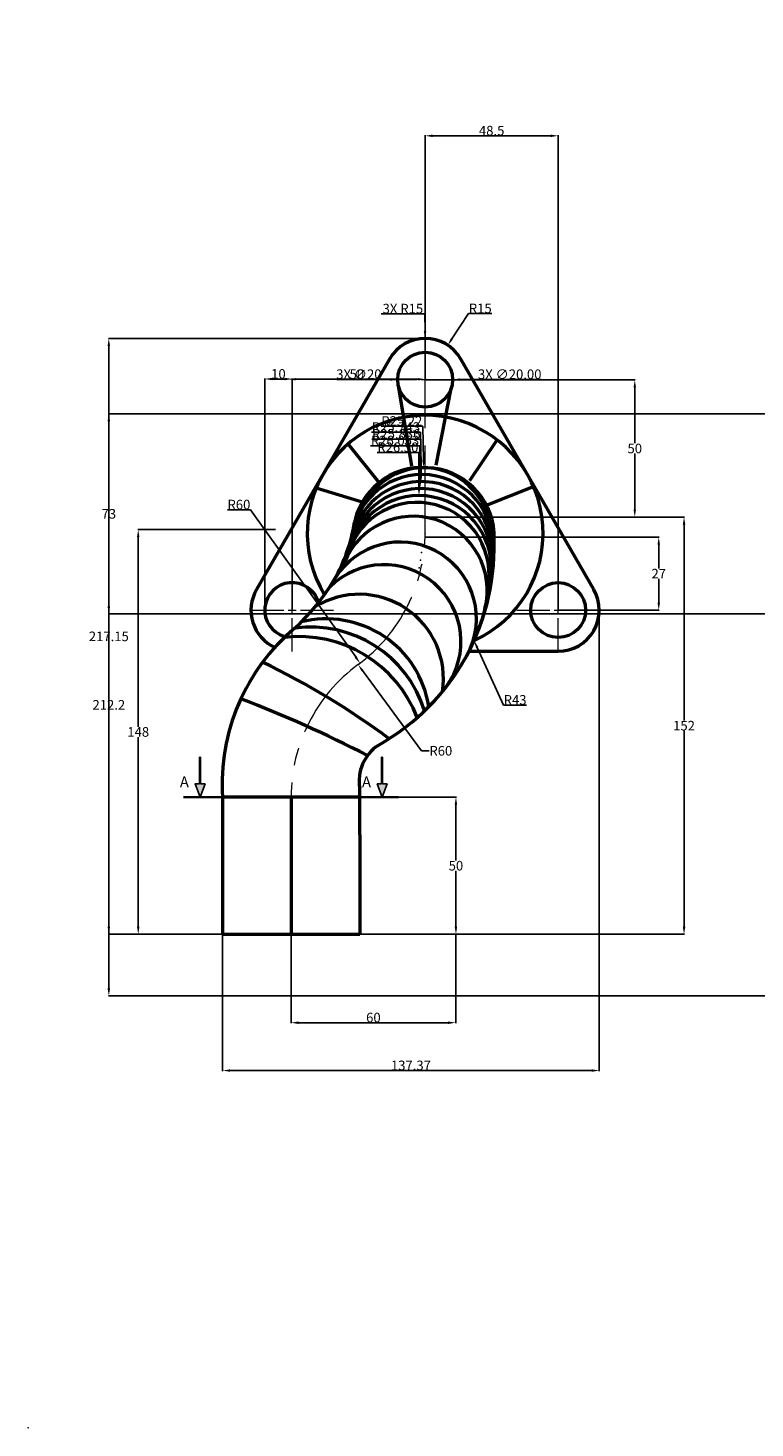
# Model space of a CAD drawing. Units: millimetres. Extents: x 795 to 1506, y 326 to 837.
# Tile 1 of 2: x 795 to 1060, y 326 to 837. Entities that reach past the tile are written whole.
import ezdxf

# ---------------------------------------------------------------- set-up
doc = ezdxf.new("R2010")
doc.units = ezdxf.units.MM
doc.header["$MEASUREMENT"] = 0
doc.linetypes.add('CENTER', pattern=[50.8, 31.75, -6.35, 6.35, -6.35])
doc.linetypes.add('PHANTOM', pattern=[63.5, 31.75, -6.35, 6.35, -6.35, 6.35, -6.35])
for name, color, linetype, lineweight in [('M-CNTR', 251, 'CENTER', 18), ('M-DIMS', 2, 'Continuous', 25), ('M-OUTL', 7, 'Continuous', 50), ('M-SECT', 7, 'PHANTOM', 35), ('M-SYMB', 7, 'Continuous', 25), ('M-TEXT', 7, 'Continuous', 25)]:
    doc.layers.add(name, color=color, linetype=linetype, lineweight=lineweight)
doc.styles.get("Standard").update_dxf_attribs({"font": 'arial.ttf'})
doc.dimstyles.get("Standard").update_dxf_attribs({"dimtxt": 3.5, "dimasz": 2.75, "dimexe": 0.18, "dimexo": 0.0625, "dimgap": 0.09, "dimtad": 1, "dimtih": 1, "dimtoh": 1, "dimdec": 0, "dimzin": 0, "dimdsep": 46, "dimtxsty": 'Standard', "dimcen": 0.09, "dimadec": 0, "dimazin": 0, "dimtfac": 1, "dimtdec": 0, "dimtofl": 0, "dimtmove": 0, "dimatfit": 3, "dimfxl": 1, "dimtolj": 1, "dimtzin": 0, "dimarcsym": 0})

# ---------------------------------------------------------------- blocks, each defined once
blk = doc.blocks.new('*U1')
at = {"layer": 'M-CNTR', "color": 0, "transparency": 16777216}
for p, q in [((0, 3), (0, 15.12)), ((-15.12, 0), (-3, 0)), ((3, 0), (15.12, 0)), ((0, -15.12), (0, -3))]:
    blk.add_line(p, q, dxfattribs=at)
at = {"layer": 'M-CNTR', "color": 0, "linetype": 'Continuous', "transparency": 16777216}
for p, q in [((-1.5, 0), (1.5, 0)), ((0, -1.5), (0, 1.5))]:
    blk.add_line(p, q, dxfattribs=at)
blk = doc.blocks.new('*U2')
at = {"layer": 'M-CNTR', "color": 0, "transparency": 16777216}
for p, q in [((0, 3), (0, 15.12)), ((-15.12, 0), (-3, 0)), ((3, 0), (15.12, 0)), ((0, -15.12), (0, -3))]:
    blk.add_line(p, q, dxfattribs=at)
at = {"layer": 'M-CNTR', "color": 0, "linetype": 'Continuous', "transparency": 16777216}
for p, q in [((-1.5, 0), (1.5, 0)), ((0, -1.5), (0, 1.5))]:
    blk.add_line(p, q, dxfattribs=at)
blk = doc.blocks.new('*U3')
at = {"layer": 'M-CNTR', "color": 0, "transparency": 16777216}
for p, q in [((0, 3), (0, 15.12)), ((-15.12, 0), (-3, 0)), ((3, 0), (15.12, 0)), ((0, -15.12), (0, -3))]:
    blk.add_line(p, q, dxfattribs=at)
at = {"layer": 'M-CNTR', "color": 0, "linetype": 'Continuous', "transparency": 16777216}
for p, q in [((-1.5, 0), (1.5, 0)), ((0, -1.5), (0, 1.5))]:
    blk.add_line(p, q, dxfattribs=at)
blk = doc.blocks.new('*D8')
at = {"layer": 'Defpoints', "color": 0, "transparency": 16777216}
for p in [(834.94, 653.74), (885.07, 653.74), (865.68, 506.24)]:
    blk.add_point(p, dxfattribs=at)
at = {"layer": 'M-DIMS', "color": 0, "lineweight": -2, "transparency": 16777216}
for p, q in [((885, 653.74), (834.76, 653.74)), ((834.94, 650.99), (834.94, 581.87)), ((834.94, 508.99), (834.94, 578.12)), ((865.61, 506.24), (834.76, 506.24))]:
    blk.add_line(p, q, dxfattribs=at)
at = {"layer": 'M-DIMS', "color": 0, "transparency": 16777216}
for points in [[(834.49, 650.99), (835.4, 650.99), (834.94, 653.74)], [(834.49, 508.99), (835.4, 508.99), (834.94, 506.24)]]:
    blk.add_solid(points, dxfattribs=at)
at = {"layer": 'M-DIMS', "color": 0, "transparency": 16777216, "insert": (834.94, 579.99), "char_height": 3.5, "attachment_point": 5}
blk.add_mtext('\\A1;148', dxfattribs=at)
blk = doc.blocks.new('*D9')
at = {"layer": 'Defpoints', "color": 0, "transparency": 16777216}
for p in [(881.05, 708.62), (881.05, 624.39), (891.05, 624.39)]:
    blk.add_point(p, dxfattribs=at)
at = {"layer": 'M-DIMS', "color": 0, "lineweight": -2, "transparency": 16777216}
for p, q in [((881.05, 624.46), (881.05, 708.8)), ((888.3, 708.62), (883.8, 708.62)), ((891.05, 624.46), (891.05, 708.8))]:
    blk.add_line(p, q, dxfattribs=at)
at = {"layer": 'M-DIMS', "color": 0, "transparency": 16777216}
for points in [[(883.8, 709.07), (883.8, 708.16), (881.05, 708.62)], [(888.3, 709.07), (888.3, 708.16), (891.05, 708.62)]]:
    blk.add_solid(points, dxfattribs=at)
at = {"layer": 'M-DIMS', "color": 0, "transparency": 16777216, "insert": (886.05, 710.49), "char_height": 3.5, "attachment_point": 5}
blk.add_mtext('\\A1;10', dxfattribs=at)
blk = doc.blocks.new('*D10')
at = {"layer": 'Defpoints', "color": 0, "transparency": 16777216}
for p in [(947.78, 720.93), (939.55, 708.39)]:
    blk.add_point(p, dxfattribs=at)
at = {"layer": 'M-DIMS', "color": 0, "lineweight": -2, "transparency": 16777216}
for p, q in [((955.36, 732.49), (949.29, 723.23)), ((963.84, 732.49), (955.36, 732.49)), ((939.46, 708.39), (939.64, 708.39)), ((939.55, 708.3), (939.55, 708.48))]:
    blk.add_line(p, q, dxfattribs=at)
at = {"layer": 'M-DIMS', "color": 0, "transparency": 16777216}
blk.add_solid([(948.9, 723.48), (949.67, 722.98), (947.78, 720.93)], dxfattribs=at)
at = {"layer": 'M-DIMS', "color": 0, "transparency": 16777216, "insert": (959.64, 734.36), "char_height": 3.5, "attachment_point": 5}
blk.add_mtext('\\A1;R15', dxfattribs=at)
blk = doc.blocks.new('*D11')
at = {"layer": 'Defpoints', "color": 0, "transparency": 16777216}
for p in [(889.64, 708.52), (889.64, 708.39), (939.64, 708.39)]:
    blk.add_point(p, dxfattribs=at)
at = {"layer": 'M-DIMS', "color": 0, "lineweight": -2, "transparency": 16777216}
for p, q in [((889.64, 708.46), (889.64, 708.7)), ((936.89, 708.52), (892.39, 708.52)), ((939.64, 708.46), (939.64, 708.7))]:
    blk.add_line(p, q, dxfattribs=at)
at = {"layer": 'M-DIMS', "color": 0, "transparency": 16777216}
for points in [[(892.39, 708.98), (892.39, 708.06), (889.64, 708.52)], [(936.89, 708.98), (936.89, 708.06), (939.64, 708.52)]]:
    blk.add_solid(points, dxfattribs=at)
at = {"layer": 'M-DIMS', "color": 0, "transparency": 16777216, "insert": (914.64, 710.4), "char_height": 3.5, "attachment_point": 5}
blk.add_mtext('\\A1;50', dxfattribs=at)
blk = doc.blocks.new('*D12')
at = {"layer": 'Defpoints', "color": 0, "transparency": 16777216}
for p in [(915.08, 604.54), (950.68, 556.24)]:
    blk.add_point(p, dxfattribs=at)
at = {"layer": 'M-DIMS', "color": 0, "lineweight": -2, "transparency": 16777216}
for p, q in [((938.24, 573.11), (916.71, 602.33)), ((940.99, 573.11), (938.24, 573.11))]:
    blk.add_line(p, q, dxfattribs=at)
at = {"layer": 'M-DIMS', "color": 0, "transparency": 16777216}
blk.add_solid([(917.08, 602.6), (916.34, 602.06), (915.08, 604.54)], dxfattribs=at)
at = {"layer": 'M-DIMS', "color": 0, "transparency": 16777216, "insert": (945.26, 573.11), "char_height": 3.5, "attachment_point": 5}
blk.add_mtext('\\A1;R60', dxfattribs=at)
blk = doc.blocks.new('*D13')
at = {"layer": 'Defpoints', "color": 0, "transparency": 16777216}
for p in [(939.52, 650.96), (1024.71, 650.96), (988.04, 624.39)]:
    blk.add_point(p, dxfattribs=at)
at = {"layer": 'M-DIMS', "color": 0, "lineweight": -2, "transparency": 16777216}
for p, q in [((939.58, 650.96), (1024.89, 650.96)), ((1024.71, 648.21), (1024.71, 639.52)), ((1024.71, 627.14), (1024.71, 635.83)), ((988.11, 624.39), (1024.89, 624.39))]:
    blk.add_line(p, q, dxfattribs=at)
at = {"layer": 'M-DIMS', "color": 0, "transparency": 16777216}
for points in [[(1024.25, 648.21), (1025.17, 648.21), (1024.71, 650.96)], [(1024.25, 627.14), (1025.17, 627.14), (1024.71, 624.39)]]:
    blk.add_solid(points, dxfattribs=at)
at = {"layer": 'M-DIMS', "color": 0, "transparency": 16777216, "insert": (1024.71, 637.68), "char_height": 3.5, "attachment_point": 5}
blk.add_mtext('\\A1;27', dxfattribs=at)
blk = doc.blocks.new('*D14')
at = {"layer": 'Defpoints', "color": 0, "transparency": 16777216}
for p in [(939.55, 708.3), (939.55, 658.3), (1015.97, 658.3)]:
    blk.add_point(p, dxfattribs=at)
at = {"layer": 'M-DIMS', "color": 0, "lineweight": -2, "transparency": 16777216}
for p, q in [((939.61, 708.3), (1016.15, 708.3)), ((1015.97, 705.55), (1015.97, 685.18)), ((1015.97, 661.05), (1015.97, 681.43)), ((939.61, 658.3), (1016.15, 658.3))]:
    blk.add_line(p, q, dxfattribs=at)
at = {"layer": 'M-DIMS', "color": 0, "transparency": 16777216}
for points in [[(1015.51, 705.55), (1016.42, 705.55), (1015.97, 708.3)], [(1015.51, 661.05), (1016.42, 661.05), (1015.97, 658.3)]]:
    blk.add_solid(points, dxfattribs=at)
at = {"layer": 'M-DIMS', "color": 0, "transparency": 16777216, "insert": (1015.97, 683.3), "char_height": 3.5, "attachment_point": 5}
blk.add_mtext('\\A1;50', dxfattribs=at)
blk = doc.blocks.new('*D15')
at = {"layer": 'Defpoints', "color": 0, "transparency": 16777216}
for p in [(939.55, 658.3), (950.68, 506.24), (1033.93, 506.24)]:
    blk.add_point(p, dxfattribs=at)
at = {"layer": 'M-DIMS', "color": 0, "lineweight": -2, "transparency": 16777216}
for p, q in [((939.61, 658.3), (1034.11, 658.3)), ((1033.93, 655.55), (1033.93, 584.15)), ((1033.93, 508.99), (1033.93, 580.4)), ((950.74, 506.24), (1034.11, 506.24))]:
    blk.add_line(p, q, dxfattribs=at)
at = {"layer": 'M-DIMS', "color": 0, "transparency": 16777216}
for points in [[(1033.47, 655.55), (1034.39, 655.55), (1033.93, 658.3)], [(1033.47, 508.99), (1034.39, 508.99), (1033.93, 506.24)]]:
    blk.add_solid(points, dxfattribs=at)
at = {"layer": 'M-DIMS', "color": 0, "transparency": 16777216, "insert": (1033.93, 582.27), "char_height": 3.5, "attachment_point": 5}
blk.add_mtext('\\A1;152', dxfattribs=at)
blk = doc.blocks.new('*D18')
at = {"layer": 'Defpoints', "color": 0, "transparency": 16777216}
for p in [(890.68, 506.24), (950.68, 506.24), (950.68, 474)]:
    blk.add_point(p, dxfattribs=at)
at = {"layer": 'M-DIMS', "color": 0, "lineweight": -2, "transparency": 16777216}
for p, q in [((890.68, 506.18), (890.68, 473.82)), ((950.68, 506.18), (950.68, 473.82)), ((893.43, 474), (947.93, 474))]:
    blk.add_line(p, q, dxfattribs=at)
at = {"layer": 'M-DIMS', "color": 0, "transparency": 16777216}
for points in [[(893.43, 474.46), (893.43, 473.54), (890.68, 474)], [(947.93, 474.46), (947.93, 473.54), (950.68, 474)]]:
    blk.add_solid(points, dxfattribs=at)
at = {"layer": 'M-DIMS', "color": 0, "transparency": 16777216, "insert": (920.68, 475.88), "char_height": 3.5, "attachment_point": 5}
blk.add_mtext('\\A1;60', dxfattribs=at)
blk = doc.blocks.new('*D19')
at = {"layer": 'Defpoints', "color": 0, "transparency": 16777216}
for p in [(915.81, 605.08), (950.68, 556.24)]:
    blk.add_point(p, dxfattribs=at)
at = {"layer": 'M-DIMS', "color": 0, "lineweight": -2, "transparency": 16777216}
for p, q in [((867.47, 660.97), (875.91, 660.97)), ((875.91, 660.97), (914.22, 607.32)), ((950.59, 556.24), (950.77, 556.24)), ((950.68, 556.15), (950.68, 556.33))]:
    blk.add_line(p, q, dxfattribs=at)
blk.add_arc((950.68, 556.24), 60, 125.3513, 126.2918, dxfattribs=at)
at = {"layer": 'M-DIMS', "color": 0, "transparency": 16777216}
blk.add_solid([(914.59, 607.58), (913.84, 607.05), (915.81, 605.08)], dxfattribs=at)
at = {"layer": 'M-DIMS', "color": 0, "transparency": 16777216, "insert": (871.65, 662.85), "char_height": 3.5, "attachment_point": 5}
blk.add_mtext('\\A1;R60', dxfattribs=at)
blk = doc.blocks.new('*D20')
at = {"layer": 'Defpoints', "color": 0, "transparency": 16777216}
for p in [(915.68, 556.24), (950.77, 556.24), (915.68, 506.24)]:
    blk.add_point(p, dxfattribs=at)
at = {"layer": 'M-DIMS', "color": 0, "lineweight": -2, "transparency": 16777216}
for p, q in [((915.74, 556.24), (950.95, 556.24)), ((950.77, 553.49), (950.77, 533.12)), ((950.77, 508.99), (950.77, 529.37)), ((915.74, 506.24), (950.95, 506.24))]:
    blk.add_line(p, q, dxfattribs=at)
at = {"layer": 'M-DIMS', "color": 0, "transparency": 16777216}
for points in [[(950.31, 553.49), (951.22, 553.49), (950.77, 556.24)], [(950.31, 508.99), (951.22, 508.99), (950.77, 506.24)]]:
    blk.add_solid(points, dxfattribs=at)
at = {"layer": 'M-DIMS', "color": 0, "transparency": 16777216, "insert": (950.77, 531.24), "char_height": 3.5, "attachment_point": 5}
blk.add_mtext('\\A1;50', dxfattribs=at)
blk = doc.blocks.new('*D21')
at = {"layer": 'Defpoints', "color": 0, "transparency": 16777216}
for p in [(988.04, 797.27), (939.55, 708.39), (988.04, 624.39)]:
    blk.add_point(p, dxfattribs=at)
at = {"layer": 'M-DIMS', "color": 0, "lineweight": -2, "transparency": 16777216}
for p, q in [((939.55, 708.46), (939.55, 797.45)), ((942.3, 797.27), (985.29, 797.27)), ((988.04, 624.46), (988.04, 797.45))]:
    blk.add_line(p, q, dxfattribs=at)
at = {"layer": 'M-DIMS', "color": 0, "transparency": 16777216}
for points in [[(942.3, 797.72), (942.3, 796.81), (939.55, 797.27)], [(985.29, 797.72), (985.29, 796.81), (988.04, 797.27)]]:
    blk.add_solid(points, dxfattribs=at)
at = {"layer": 'M-DIMS', "color": 0, "transparency": 16777216, "insert": (963.8, 799.14), "char_height": 3.5, "attachment_point": 5}
blk.add_mtext('\\A1;48.5', dxfattribs=at)
blk = doc.blocks.new('*D22')
at = {"layer": 'Defpoints', "color": 0, "transparency": 16777216}
for p in [(1003.04, 624.39), (865.68, 506.24), (1003.04, 456.57)]:
    blk.add_point(p, dxfattribs=at)
at = {"layer": 'M-DIMS', "color": 0, "lineweight": -2, "transparency": 16777216}
for p, q in [((1003.04, 624.33), (1003.04, 456.39)), ((865.68, 506.18), (865.68, 456.39)), ((868.43, 456.57), (1000.29, 456.57))]:
    blk.add_line(p, q, dxfattribs=at)
at = {"layer": 'M-DIMS', "color": 0, "transparency": 16777216}
for points in [[(868.43, 457.02), (868.43, 456.11), (865.68, 456.57)], [(1000.29, 457.02), (1000.29, 456.11), (1003.04, 456.57)]]:
    blk.add_solid(points, dxfattribs=at)
at = {"layer": 'M-DIMS', "color": 0, "transparency": 16777216, "insert": (934.36, 458.44), "char_height": 3.5, "attachment_point": 5}
blk.add_mtext('\\A1;137.37', dxfattribs=at)
blk = doc.blocks.new('*D23')
at = {"layer": 'Defpoints', "color": 0, "transparency": 16777216}
for p in [(824.22, 723.39), (939.55, 723.39), (865.68, 506.24)]:
    blk.add_point(p, dxfattribs=at)
at = {"layer": 'M-DIMS', "color": 0, "lineweight": -2, "transparency": 16777216}
for p, q in [((939.48, 723.39), (824.04, 723.39)), ((824.22, 720.64), (824.22, 616.7)), ((824.22, 508.99), (824.22, 612.94)), ((865.61, 506.24), (824.04, 506.24))]:
    blk.add_line(p, q, dxfattribs=at)
at = {"layer": 'M-DIMS', "color": 0, "transparency": 16777216}
for points in [[(823.76, 720.64), (824.68, 720.64), (824.22, 723.39)], [(823.76, 508.99), (824.68, 508.99), (824.22, 506.24)]]:
    blk.add_solid(points, dxfattribs=at)
at = {"layer": 'M-DIMS', "color": 0, "transparency": 16777216, "insert": (824.22, 614.82), "char_height": 3.5, "attachment_point": 5}
blk.add_mtext('\\A1;217.15', dxfattribs=at)
blk = doc.blocks.new('*D25')
at = {"layer": 'Defpoints', "color": 0, "transparency": 16777216}
for p in [(1310.11, 695.98), (824.22, 622.98), (1265.11, 622.98)]:
    blk.add_point(p, dxfattribs=at)
at = {"layer": 'M-DIMS', "color": 0, "lineweight": -2, "transparency": 16777216}
for p, q in [((1310.05, 695.98), (824.04, 695.98)), ((824.22, 693.23), (824.22, 661.36)), ((824.22, 625.73), (824.22, 657.6)), ((1265.05, 622.98), (824.04, 622.98))]:
    blk.add_line(p, q, dxfattribs=at)
at = {"layer": 'M-DIMS', "color": 0, "transparency": 16777216}
for points in [[(823.76, 693.23), (824.68, 693.23), (824.22, 695.98)], [(823.76, 625.73), (824.68, 625.73), (824.22, 622.98)]]:
    blk.add_solid(points, dxfattribs=at)
at = {"layer": 'M-DIMS', "color": 0, "transparency": 16777216, "insert": (824.22, 659.48), "char_height": 3.5, "attachment_point": 5}
blk.add_mtext('\\A1;73', dxfattribs=at)
blk = doc.blocks.new('*D27')
at = {"layer": 'Defpoints', "color": 0, "transparency": 16777216}
for p in [(824.22, 695.98), (1310.11, 695.98), (1165.11, 483.77)]:
    blk.add_point(p, dxfattribs=at)
at = {"layer": 'M-DIMS', "color": 0, "lineweight": -2, "transparency": 16777216}
for p, q in [((1310.05, 695.98), (824.04, 695.98)), ((824.22, 693.23), (824.22, 591.72)), ((824.22, 486.52), (824.22, 588.03)), ((1165.05, 483.77), (824.04, 483.77))]:
    blk.add_line(p, q, dxfattribs=at)
at = {"layer": 'M-DIMS', "color": 0, "transparency": 16777216}
for points in [[(823.76, 693.23), (824.68, 693.23), (824.22, 695.98)], [(823.76, 486.52), (824.68, 486.52), (824.22, 483.77)]]:
    blk.add_solid(points, dxfattribs=at)
at = {"layer": 'M-DIMS', "color": 0, "transparency": 16777216, "insert": (824.22, 589.87), "char_height": 3.5, "attachment_point": 5}
blk.add_mtext('\\A1;212.2', dxfattribs=at)
blk = doc.blocks.new('*D30')
at = {"layer": 'Defpoints', "color": 0, "transparency": 16777216}
for p in [(939.5, 723.39), (939.55, 708.39)]:
    blk.add_point(p, dxfattribs=at)
at = {"layer": 'M-DIMS', "color": 0, "lineweight": -2, "transparency": 16777216}
for p, q in [((923.47, 732.39), (939.47, 732.39)), ((939.47, 732.39), (939.49, 726.14)), ((939.46, 708.39), (939.64, 708.39)), ((939.55, 708.3), (939.55, 708.48))]:
    blk.add_line(p, q, dxfattribs=at)
at = {"layer": 'M-DIMS', "color": 0, "transparency": 16777216}
blk.add_solid([(939.95, 726.14), (939.03, 726.14), (939.5, 723.39)], dxfattribs=at)
at = {"layer": 'M-DIMS', "color": 0, "transparency": 16777216, "insert": (931.43, 734.27), "char_height": 3.5, "attachment_point": 5}
blk.add_mtext('\\A1;3X R15', dxfattribs=at)
blk = doc.blocks.new('*D31')
at = {"layer": 'Defpoints', "color": 0, "transparency": 16777216}
for p in [(929.55, 708.4), (949.55, 708.39)]:
    blk.add_point(p, dxfattribs=at)
at = {"layer": 'M-DIMS', "color": 0, "lineweight": -2, "transparency": 16777216}
for p, q in [((907.32, 708.4), (923.55, 708.4)), ((923.55, 708.4), (926.8, 708.4)), ((939.46, 708.39), (939.64, 708.39)), ((939.55, 708.3), (939.55, 708.48))]:
    blk.add_line(p, q, dxfattribs=at)
at = {"layer": 'M-DIMS', "color": 0, "transparency": 16777216}
blk.add_solid([(926.8, 708.86), (926.8, 707.94), (929.55, 708.4)], dxfattribs=at)
at = {"layer": 'M-DIMS', "color": 0, "transparency": 16777216, "insert": (915.39, 710.38), "char_height": 3.5, "attachment_point": 5}
blk.add_mtext('\\A1;3X ∅20', dxfattribs=at)
blk = doc.blocks.new('*D32')
at = {"layer": 'Defpoints', "color": 0, "transparency": 16777216}
for p in [(939.55, 652.39), (957.37, 613.26)]:
    blk.add_point(p, dxfattribs=at)
at = {"layer": 'M-DIMS', "color": 0, "lineweight": -2, "transparency": 16777216}
for p, q in [((939.46, 652.39), (939.64, 652.39)), ((939.55, 652.3), (939.55, 652.48)), ((968.06, 589.78), (958.51, 610.76)), ((976.52, 589.78), (968.06, 589.78))]:
    blk.add_line(p, q, dxfattribs=at)
at = {"layer": 'M-DIMS', "color": 0, "transparency": 16777216}
blk.add_solid([(958.93, 610.95), (958.09, 610.57), (957.37, 613.26)], dxfattribs=at)
at = {"layer": 'M-DIMS', "color": 0, "transparency": 16777216, "insert": (972.34, 591.66), "char_height": 3.5, "attachment_point": 5}
blk.add_mtext('\\A1;R43', dxfattribs=at)
blk = doc.blocks.new('*D35')
at = {"layer": 'Defpoints', "color": 0, "transparency": 16777216}
for p in [(929.55, 708.4), (949.55, 708.39)]:
    blk.add_point(p, dxfattribs=at)
at = {"layer": 'M-DIMS', "color": 0, "lineweight": -2, "transparency": 16777216}
for p, q in [((939.46, 708.39), (939.64, 708.39)), ((939.55, 708.3), (939.55, 708.48)), ((958.82, 708.39), (952.3, 708.39)), ((981.85, 708.39), (958.82, 708.39))]:
    blk.add_line(p, q, dxfattribs=at)
at = {"layer": 'M-DIMS', "color": 0, "transparency": 16777216}
blk.add_solid([(952.3, 708.85), (952.3, 707.93), (949.55, 708.39)], dxfattribs=at)
at = {"layer": 'M-DIMS', "color": 0, "transparency": 16777216, "insert": (970.38, 710.36), "char_height": 3.5, "attachment_point": 5}
blk.add_mtext('\\A1;3X ∅20.00', dxfattribs=at)
blk = doc.blocks.new('*D38')
at = {"layer": 'Defpoints', "color": 0, "transparency": 16777216}
for p in [(1227.9, 642.63), (794.84, 326.38)]:
    blk.add_point(p, dxfattribs=at)
at = {"layer": 'M-DIMS', "color": 0, "lineweight": -2, "transparency": 16777216}
for p, q in [((1487.74, 832.38), (1230.12, 644.25)), ((1505.7, 832.38), (1487.74, 832.38)), ((794.75, 326.38), (794.93, 326.38)), ((794.84, 326.29), (794.84, 326.47))]:
    blk.add_line(p, q, dxfattribs=at)
at = {"layer": 'M-DIMS', "color": 0, "transparency": 16777216}
blk.add_solid([(1229.85, 644.62), (1230.39, 643.88), (1227.9, 642.63)], dxfattribs=at)
at = {"layer": 'M-DIMS', "color": 0, "transparency": 16777216, "insert": (1496.76, 834.26), "char_height": 3.5, "attachment_point": 5}
blk.add_mtext('\\A1;R536.24', dxfattribs=at)
blk = doc.blocks.new('*D48')
at = {"layer": 'Defpoints', "color": 0, "transparency": 16777216}
for p in [(939, 676.3), (939.53, 651.08)]:
    blk.add_point(p, dxfattribs=at)
at = {"layer": 'M-DIMS', "color": 0, "lineweight": -2, "transparency": 16777216}
for p, q in [((923.47, 691.43), (938.68, 691.43)), ((938.68, 691.43), (938.94, 679.05)), ((939.44, 651.08), (939.62, 651.08)), ((939.53, 650.99), (939.53, 651.17))]:
    blk.add_line(p, q, dxfattribs=at)
at = {"layer": 'M-DIMS', "color": 0, "transparency": 16777216}
blk.add_solid([(939.4, 679.06), (938.48, 679.04), (939, 676.3)], dxfattribs=at)
at = {"layer": 'M-DIMS', "color": 0, "transparency": 16777216, "insert": (931.03, 693.31), "char_height": 3.5, "attachment_point": 5}
blk.add_mtext('\\A1;R25.22', dxfattribs=at)
blk = doc.blocks.new('*D49')
at = {"layer": 'Defpoints', "color": 0, "transparency": 16777216}
for p in [(938.1, 673.79), (938.41, 648.05)]:
    blk.add_point(p, dxfattribs=at)
at = {"layer": 'M-DIMS', "color": 0, "lineweight": -2, "transparency": 16777216}
for p, q in [((919.94, 689.23), (937.91, 689.23)), ((937.91, 689.23), (938.07, 676.54)), ((938.32, 648.05), (938.5, 648.05)), ((938.41, 647.96), (938.41, 648.14))]:
    blk.add_line(p, q, dxfattribs=at)
at = {"layer": 'M-DIMS', "color": 0, "transparency": 16777216}
blk.add_solid([(938.53, 676.54), (937.61, 676.53), (938.1, 673.79)], dxfattribs=at)
at = {"layer": 'M-DIMS', "color": 0, "transparency": 16777216, "insert": (928.88, 691.11), "char_height": 3.5, "attachment_point": 5}
blk.add_mtext('\\A1;R25.743', dxfattribs=at)
blk = doc.blocks.new('*D50')
at = {"layer": 'Defpoints', "color": 0, "transparency": 16777216}
for p in [(938.1, 671.22), (938.22, 645.38)]:
    blk.add_point(p, dxfattribs=at)
at = {"layer": 'M-DIMS', "color": 0, "lineweight": -2, "transparency": 16777216}
for p, q in [((920.06, 686.72), (938.02, 686.72)), ((938.02, 686.72), (938.09, 673.97)), ((938.13, 645.38), (938.31, 645.38)), ((938.22, 645.29), (938.22, 645.47))]:
    blk.add_line(p, q, dxfattribs=at)
at = {"layer": 'M-DIMS', "color": 0, "transparency": 16777216}
blk.add_solid([(938.54, 673.97), (937.63, 673.97), (938.1, 671.22)], dxfattribs=at)
at = {"layer": 'M-DIMS', "color": 0, "transparency": 16777216, "insert": (929, 688.6), "char_height": 3.5, "attachment_point": 5}
blk.add_mtext('\\A1;R25.836', dxfattribs=at)
blk = doc.blocks.new('*D51')
at = {"layer": 'Defpoints', "color": 0, "transparency": 16777216}
for p in [(937.7, 668.66), (937.86, 642.61)]:
    blk.add_point(p, dxfattribs=at)
at = {"layer": 'M-DIMS', "color": 0, "lineweight": -2, "transparency": 16777216}
for p, q in [((919.64, 684.29), (937.61, 684.29)), ((937.61, 684.29), (937.68, 671.41)), ((937.77, 642.61), (937.95, 642.61)), ((937.86, 642.52), (937.86, 642.7))]:
    blk.add_line(p, q, dxfattribs=at)
at = {"layer": 'M-DIMS', "color": 0, "transparency": 16777216}
blk.add_solid([(938.14, 671.41), (937.23, 671.41), (937.7, 668.66)], dxfattribs=at)
at = {"layer": 'M-DIMS', "color": 0, "transparency": 16777216, "insert": (928.58, 686.17), "char_height": 3.5, "attachment_point": 5}
blk.add_mtext('\\A1;R26.053', dxfattribs=at)
blk = doc.blocks.new('*D52')
at = {"layer": 'Defpoints', "color": 0, "transparency": 16777216}
for p in [(937.3, 666.11), (937.38, 639.81)]:
    blk.add_point(p, dxfattribs=at)
at = {"layer": 'M-DIMS', "color": 0, "lineweight": -2, "transparency": 16777216}
for p, q in [((922.01, 681.89), (937.25, 681.89)), ((937.25, 681.89), (937.29, 668.86)), ((937.29, 639.81), (937.47, 639.81)), ((937.38, 639.72), (937.38, 639.9))]:
    blk.add_line(p, q, dxfattribs=at)
at = {"layer": 'M-DIMS', "color": 0, "transparency": 16777216}
blk.add_solid([(937.75, 668.86), (936.83, 668.86), (937.3, 666.11)], dxfattribs=at)
at = {"layer": 'M-DIMS', "color": 0, "transparency": 16777216, "insert": (929.59, 683.77), "char_height": 3.5, "attachment_point": 5}
blk.add_mtext('\\A1;R26.30', dxfattribs=at)

msp = doc.modelspace()

# ---------------------------------------------------------------- hatches: boundary and pattern name
at = {"layer": 'M-SYMB'}
h = msp.add_hatch(color=256, dxfattribs=at)
h.dxf.hatch_style = 1
h.paths.add_polyline_path([(925.6898, 561.0326), (924.0378, 561.0326), (924.0378, 570.8173), (923.6718, 570.8173), (923.6718, 561.0326), (922.062, 561.0326), (923.8759, 556.2447)])
h.paths.add_polyline_path([(859.2832, 561.0326), (857.6311, 561.0326), (857.6311, 570.8173), (857.2651, 570.8173), (857.2651, 561.0326), (855.6553, 561.0326), (857.4692, 556.2447)])

# ---------------------------------------------------------------- linework, layer by layer
at = {"layer": 'M-CNTR'}
for p, q in [((939.5474, 652.6424), (939.5474, 708.3926)), ((939.5474, 652.3926), (939.5474, 652.8922))]:
    msp.add_line(p, q, dxfattribs=at)
msp.add_lwpolyline([(890.6759, 556.2447, -0.23845716), (915.1117, 604.5685, 0.23845716), (939.5474, 652.8922)], format="xyb", dxfattribs=at)
at = {"layer": 'M-OUTL'}
for p, q in [((934.6771, 676.9136), (929.959, 705.5534)), ((943.5036, 677.2119), (949.0283, 705.2125)), ((922.7488, 670.9077), (911.5244, 685.0072)), ((955.8718, 671.6751), (965.8206, 686.4326)), ((916.5519, 663.7049), (899.8152, 668.8349)), ((961.9063, 662.6126), (979.037, 669.4094)), ((915.6759, 556.2447), (865.6759, 556.2447)), ((865.6759, 556.2447), (865.6759, 506.2447)), ((890.6759, 556.2447), (890.6759, 506.2447)), ((915.6759, 556.2447), (915.6759, 559.4192)), ((915.6759, 542.4266), (915.6759, 556.2447)), ((915.6759, 542.4266), (915.6759, 506.2447)), ((865.6759, 506.2447), (890.6759, 506.2447)), ((890.6759, 506.2447), (915.6759, 506.2447))]:
    msp.add_line(p, q, dxfattribs=at)
for points in [[(926.557, 715.8926), (878.0596, 631.8926)], [(1001.0352, 631.8926), (952.5378, 715.8926)], [(955.5102, 609.3926), (988.0448, 609.3926)]]:
    msp.add_lwpolyline(points, dxfattribs=at)
for centre in [(939.5474, 708.3926), (988.0448, 624.3926)]:
    msp.add_circle(centre, 10, dxfattribs=at)
for centre, radius, start, end in [((939.5474, 708.3926), 15, 30, 150), ((939.5474, 652.3926), 43, 294.511404, 211.365853), ((938.4121, 648.0462), 25.7431, 355.008158, 173.060611), ((938.427, 651.1518), 25.221, 358.087452, 172.360995), ((939.5338, 651.0838), 25.221, 358.087452, 168.215221), ((937.8587, 642.6094), 26.0529, 352.229151, 168.41103), ((938.225, 645.3843), 25.836, 353.834249, 167.723378), ((936.6113, 637.4038), 26.2401, 347.154285, 162.831379), ((937.3815, 639.8118), 26.3008, 351.256007, 166.39452), ((935.1607, 631.5699), 27.034, 345.637808, 157.753792), ((840.3545, 674.4951), 76.6954, 312.305582, 346.226279), ((854.4504, 665.5241), 60, 330.087346, 351.15929), ((930.3934, 621.3228), 27.8537, 337.480549, 147.380148), ((881.9702, 647.2878), 82.7348, 299.229262, 3.537442), ((885.5005, 645.1754), 78.6243, 328.462297, 5.359991), ((924.584, 612.9393), 28.0233, 323.921513, 134.661478), ((891.05, 624.3926), 10, 15.840014, 254.119614), ((891.05, 624.3926), 15, 150, 245.107437), ((915.5428, 599.4869), 30.659, 350.927421, 121.756512), ((988.0448, 624.3926), 15, 270, 30), ((939.8449, 560.9265), 74.3166, 130.09884, 183.611852), ((897.9207, 574.8798), 43.3038, 17.135081, 97.889047), ((903.5423, 583.4113), 37.7738, 8.795928, 104.038853), ((893.5954, 568.5585), 46.1995, 21.148888, 96.594519), ((939.5474, 652.3926), 43, 294.460389, 294.511404), ((756.5478, 348.192), 285.409, 53.46758, 64.306195), ((713.2172, 174.4469), 446.8839, 62.647323, 69.139042), ((931.4213, 561.9562), 15.9484, 124.578012, 189.153339)]:
    msp.add_arc(centre, radius, start, end, dxfattribs=at)
at = {"layer": 'M-SECT'}
for p, q in [((865.6759, 556.2447), (851.4181, 556.2447)), ((915.6759, 556.2447), (929.8759, 556.2447))]:
    msp.add_line(p, q, dxfattribs=at)
at = {"layer": 'M-SYMB'}
for p, q in [((857.4692, 570.8173), (857.2651, 570.8173)), ((857.2651, 570.8173), (857.6311, 570.8173)), ((857.2651, 570.8173), (857.2651, 561.0326)), ((857.6311, 570.8173), (857.6311, 561.0326)), ((923.8759, 570.8173), (923.6718, 570.8173)), ((923.6718, 570.8173), (924.0378, 570.8173)), ((923.6718, 570.8173), (923.6718, 561.0326)), ((924.0378, 570.8173), (924.0378, 561.0326))]:
    msp.add_line(p, q, dxfattribs=at)
for points in [[(857.2651, 561.0326), (855.6553, 561.0326), (857.4692, 556.2447), (859.2832, 561.0326), (857.6311, 561.0326)], [(923.6718, 561.0326), (922.062, 561.0326), (923.8759, 556.2447), (925.6898, 561.0326), (924.0378, 561.0326)]]:
    msp.add_lwpolyline(points, dxfattribs=at)

# ---------------------------------------------------------------- block references
at = {"layer": 'M-CNTR'}
for name, p in [('*U3', (939.5474, 708.3926)), ('*U2', (891.05, 624.3926)), ('*U1', (988.0448, 624.3926))]:
    msp.add_blockref(name, p, dxfattribs=at)

# ---------------------------------------------------------------- texts
at = {"layer": 'M-TEXT', "char_height": 4, "attachment_point": 1}
for insert in [(850.0965, 563.7478), (916.5032, 563.7478)]:
    msp.add_mtext_dynamic_manual_height_columns('A', width=7.732083, gutter_width=1, heights=[0], dxfattribs=dict(at, insert=insert))

# ---------------------------------------------------------------- dimensions: what is measured, and where the dimension line sits
at = {"layer": 'M-DIMS'}
for center, mpoint, override, picture, middle in [((794.8393, 326.3773), (1227.9024, 642.6287), {"dimdec": 2, "dimlfac": 1, "dimrnd": 0, "dimzin": 0, "dimdsep": 46, "dimlunit": 2}, '*D38', (1496.7629, 832.3796)), ((939.5474, 708.3926), (947.7774, 720.9333), {"dimclrd": 0, "dimclre": 0, "dimclrt": 0}, '*D10', (959.6439, 732.4863)), ((939.5338, 651.0838), (939, 676.2992), {"dimdec": 2, "dimlfac": 1, "dimrnd": 0, "dimzin": 0, "dimdsep": 46, "dimlunit": 2}, '*D48', (931.0275, 691.4284)), ((938.4121, 648.0462), (938.1002, 673.7873), {"dimdec": 3, "dimlfac": 1, "dimrnd": 0, "dimzin": 0, "dimdsep": 46, "dimlunit": 2}, '*D49', (928.8832, 689.2321)), ((938.225, 645.3843), (938.0999, 671.22), {"dimdec": 3, "dimlfac": 1, "dimrnd": 0, "dimzin": 0, "dimdsep": 46, "dimlunit": 2}, '*D50', (928.9962, 686.7215)), ((937.8587, 642.6094), (937.7002, 668.6618), {"dimdec": 3, "dimlfac": 1, "dimrnd": 0, "dimzin": 0, "dimdsep": 46, "dimlunit": 2}, '*D51', (928.5754, 684.2932)), ((937.3815, 639.8118), (937.3, 666.1125), {"dimdec": 2, "dimlfac": 1, "dimrnd": 0, "dimzin": 0, "dimdsep": 46, "dimlunit": 2}, '*D52', (929.5869, 681.8929)), ((950.6759, 556.2447), (915.814, 605.0776), {"dimclrd": 0, "dimclre": 0, "dimclrt": 0}, '*D19', (871.6459, 660.9708)), ((939.5474, 652.3926), (957.37, 613.2601), {"dimdec": 0, "dimlfac": 1, "dimrnd": 0, "dimzin": 0, "dimdsep": 46, "dimlunit": 2}, '*D32', (972.3351, 589.7805)), ((950.6759, 556.2447), (915.0792, 604.5446), {"dimclrd": 0, "dimclre": 0, "dimclrt": 0}, '*D12', (945.2584, 573.1148))]:
    dim = msp.add_radius_dim(center=center, mpoint=mpoint, dimstyle='Standard', override=override, dxfattribs=at)
    dim.commit()
    dim.dimension.update_dxf_attribs({"geometry": picture, "text_midpoint": middle, "dimtype": 164})
for base, p1, p2, override, picture, middle in [((988.0448, 797.2665), (939.5474, 708.3926), (988.0448, 624.3926), {"dimdec": 1, "dimlfac": 1, "dimrnd": 0, "dimzin": 0, "dimdsep": 46, "dimlunit": 2}, '*D21', (963.7961, 799.1435)), ((889.6374, 708.5219), (939.6374, 708.3926), (889.6374, 708.3926), {"dimclrd": 0, "dimclre": 0, "dimclrt": 0}, '*D11', (914.6374, 710.3989)), ((1003.0448, 456.5661), (865.6759, 506.2447), (1003.0448, 624.3926), {"dimdec": 2, "dimlfac": 1, "dimrnd": 0, "dimzin": 0, "dimdsep": 46, "dimlunit": 2}, '*D22', (934.3604, 458.4443)), ((950.6759, 474.0029), (890.6759, 506.2447), (950.6759, 506.2447), {"dimclrd": 0, "dimclre": 0, "dimclrt": 0}, '*D18', (920.6759, 475.8799))]:
    dim = msp.add_linear_dim(base=base, p1=p1, p2=p2, dimstyle='Standard', override=override, dxfattribs=at)
    dim.commit()
    dim.dimension.update_dxf_attribs({"geometry": picture, "text_midpoint": middle})
dim = msp.add_radius_dim(center=(939.5474, 708.3926), mpoint=(939.5, 723.3926), text='3X <>', dimstyle='Standard', override={"dimdec": 0, "dimlfac": 1, "dimrnd": 0, "dimzin": 0, "dimdsep": 46, "dimlunit": 2}, dxfattribs=at)
dim.commit()
dim.dimension.update_dxf_attribs({"geometry": '*D30', "text_midpoint": (931.4278, 732.3925), "dimtype": 164})
for base, p1, p2, override, picture, middle in [((824.2181, 723.3926), (865.6759, 506.2447), (939.5474, 723.3926), {"dimdec": 2, "dimlfac": 1, "dimrnd": 0, "dimzin": 0, "dimdsep": 46, "dimlunit": 2}, '*D23', (824.2181, 614.8187)), ((1015.9662, 658.3026), (939.5474, 708.3026), (939.5474, 658.3026), {"dimclrd": 0, "dimclre": 0, "dimclrt": 0}, '*D14', (1015.9662, 683.3026)), ((824.2181, 695.9815), (1165.1104, 483.7661), (1310.1104, 695.9815), {"dimdec": 1, "dimlfac": 1, "dimrnd": 0, "dimzin": 0, "dimdsep": 46, "dimlunit": 2}, '*D27', (824.2181, 589.8738)), ((824.2181, 622.9815), (1310.1104, 695.9815), (1265.1104, 622.9815), {"dimdec": 0, "dimlfac": 1, "dimrnd": 0, "dimzin": 0, "dimdsep": 46, "dimlunit": 2}, '*D25', (824.2181, 659.4815)), ((1033.9289, 506.2447), (939.5474, 658.3026), (950.6759, 506.2447), {"dimclrd": 0, "dimclre": 0, "dimclrt": 0}, '*D15', (1033.9289, 582.2737)), ((834.9436793835, 653.7447357273), (865.6759264572, 506.2447357273), (885.0672822338, 653.7447357273), {"dimclrd": 0, "dimclre": 0, "dimclrt": 0}, '*D8', (834.9436793835, 579.9947357273)), ((1024.7077, 650.9579), (988.0448, 624.3926), (939.5162, 650.9579), {"dimclrd": 0, "dimclre": 0, "dimclrt": 0}, '*D13', (1024.7077, 637.6753)), ((950.7659, 556.2447), (915.6759, 506.2447), (915.6759, 556.2447), {"dimclrd": 0, "dimclre": 0, "dimclrt": 0}, '*D20', (950.7659, 531.2447))]:
    dim = msp.add_linear_dim(base=base, p1=p1, p2=p2, angle=90, dimstyle='Standard', override=override, dxfattribs=at)
    dim.commit()
    dim.dimension.update_dxf_attribs({"geometry": picture, "text_midpoint": middle})
dim = msp.add_diameter_dim_2p(p1=(949.5474, 708.3853), p2=(929.5474, 708.4), text='3X <>', dimstyle='Standard', override={"dimdec": 0, "dimlfac": 1, "dimrnd": 0, "dimzin": 0, "dimdsep": 46, "dimlunit": 2}, dxfattribs=at)
dim.commit()
dim.dimension.update_dxf_attribs({"geometry": '*D31', "text_midpoint": (923.5474, 708.4044), "dimtype": 163})
dim = msp.add_diameter_dim_2p(p1=(929.5474, 708.3953), p2=(949.5474, 708.39), text='3X <>', dimstyle='Standard', override={"dimdec": 2, "dimlfac": 1, "dimrnd": 0, "dimzin": 0, "dimdsep": 46, "dimlunit": 2}, dxfattribs=at)
dim.commit()
dim.dimension.update_dxf_attribs({"geometry": '*D35', "text_midpoint": (958.8172, 708.3876)})
dim = msp.add_linear_dim(base=(881.05, 708.6161), p1=(891.05, 624.3926), p2=(881.05, 624.3926), dimstyle='Standard', override={"dimclrd": 0, "dimclre": 0, "dimclrt": 0}, dxfattribs=at)
dim.commit()
dim.dimension.update_dxf_attribs({"geometry": '*D9', "text_midpoint": (886.05, 708.6161), "dimtype": 160})

doc.saveas('drawing.dxf')
